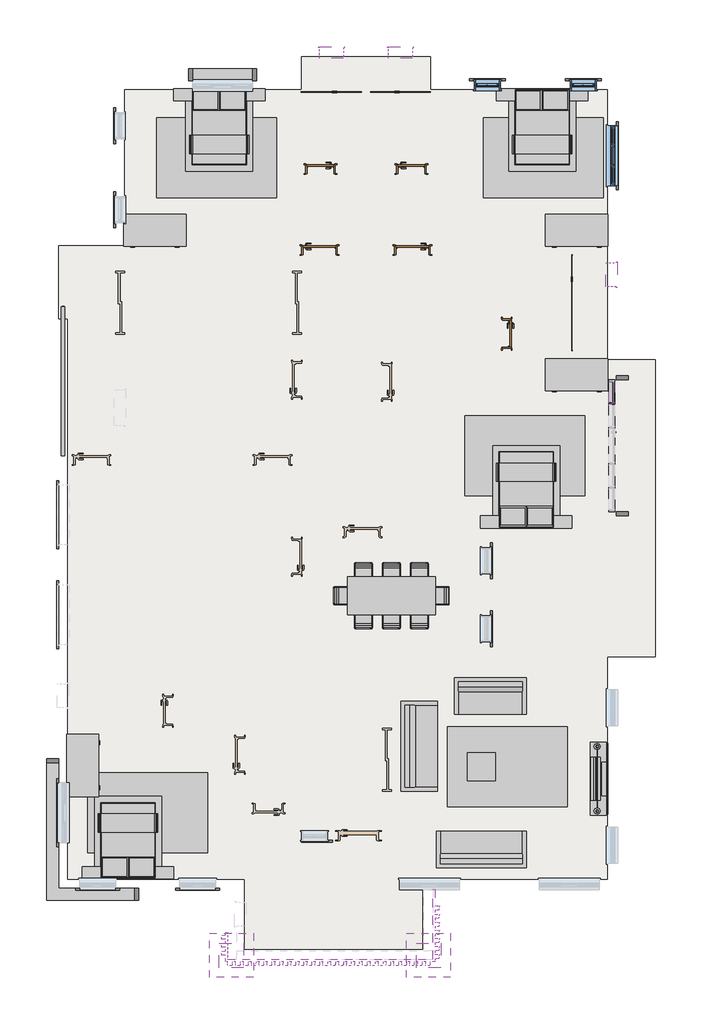
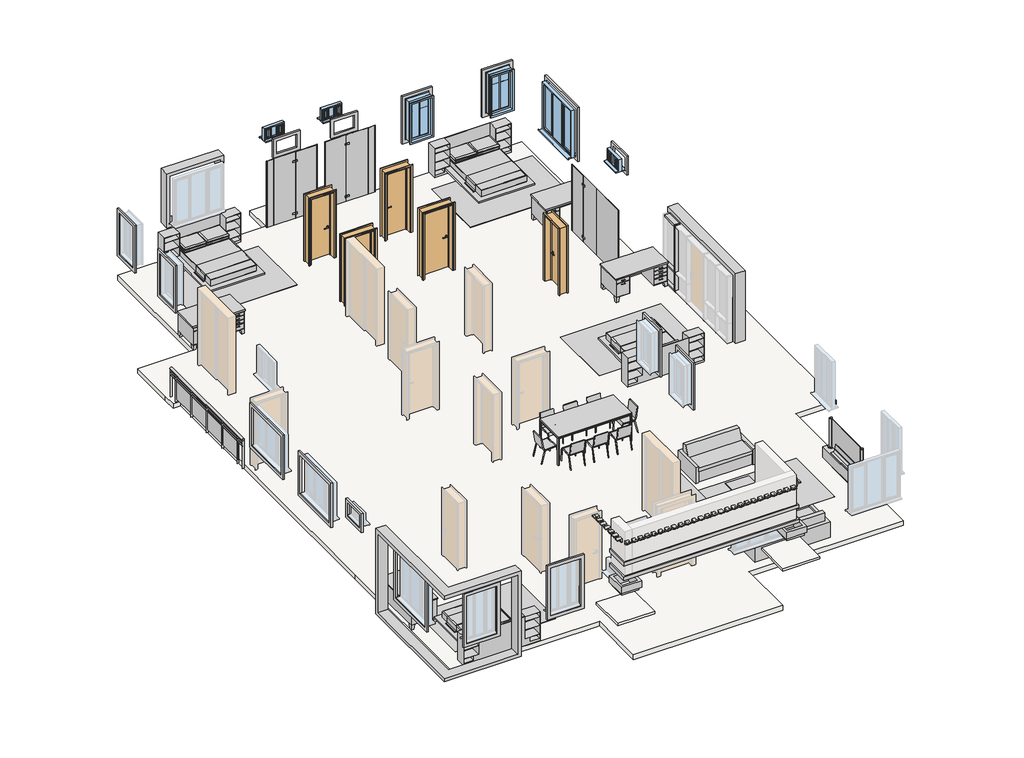
# One storey, part 2 of 2: 20 furniture elements, 6 members, 6 windows, 5 doors, 4 proxies, 3 flow terminals, 3 slabs, 1 railing.
"""IFC4 building model written with IfcOpenShell, lengths in millimetres."""

from ifc_helpers import new_model, si_unit, point, frame, origin, place, context, project, spatial, polyline, ellipse_curve, trimmed, outline, extrude, transform, mapped, element, save
from ifc_brep_helpers import plane_surface, extruded_surface, advanced_brep
from components import bed_6467_bed_6467_bd858abb, doors_intsgl_927b0b89, doors_intsgl_1caea894, doors_intsgl_900mm_doors_1c9cf9a6, doors_intsgl_900mm_doors_d21b38ee, hpl_shower_screen_rad_shower_screen_cut_corner_864de885, hpl_shower_screen_rad_shower_screen_cut_corner_ba801a97, hpl_shower_screen_rad_shower_screen_cut_corner_606f97bc, furniture_061ed33e, furniture_47c73875, furniture_703849cf, furniture_c31c7c6f, furniture_b53a9923, furniture_b3e58817, furniture_1e63cb50, casework_1_casework_1_62078cb6, casework_10_casework_10_bcdbd455, casework_3_casework_1_4875a9a3, casework_7_casework_7_7bbf8f76, casework_9_casework_9_0ee90f3f, entertainment_center_1_entertainment_center_18172_277d4ec1, m_desk_1525_x_762mm_student_8f660baf, rug1_rug_774cf3d5, rectangular_mullion_50_x_150mm_5b5377e9, rectangular_mullion_50_x_150mm_de2b7ee4, rectangular_mullion_50_x_150mm_8a69f4a4, rectangular_mullion_50_x_150mm_63369cdd, rectangular_mullion_50_x_150mm_c6835c94, tpl_plain_1500mm_wind_d4a9cd4c, tpl_plain_600mm_window_e9a44080, yu_window_casement_600x1200_84df8a12

model = new_model("IFC4")

# Units and contexts
model_context = context("Model", 3, world=origin())
ifc_project = project(units=[si_unit("LENGTHUNIT", "METRE", prefix="MILLI")], contexts=[model_context])

# Site, building, storey
site = spatial("IfcSite", under=ifc_project)
building = spatial("IfcBuilding", under=site)
storey = spatial("IfcBuildingStorey", under=building, Elevation=450.0)

# Proxies
placement = place(None, origin())
bed_6467_bed_6467_shape = bed_6467_bed_6467_bd858abb(model_context)
element("IfcBuildingElementProxy", 1, Name="BED_6467 : BED_6467", ObjectType="BED_6467 : BED_6467", at=placement, inside=storey, context=model_context, shape_type="MappedRepresentation", body=[
    mapped(bed_6467_bed_6467_shape, transform((-2061.7953966, 8065.8070837, 450.0), x_axis=(1.0, 0.0, 0.0), y_axis=(0.0, 1.0, 0.0), z_axis=(0.0, 0.0, 1.0))),
])
element("IfcBuildingElementProxy", 2, Name="BED_6467 : BED_6467", ObjectType="BED_6467 : BED_6467", at=placement, inside=storey, context=model_context, shape_type="MappedRepresentation", body=[
    mapped(bed_6467_bed_6467_shape, transform((6013.2046034, 8065.8070837, 450.0), x_axis=(1.0, 0.0, 0.0), y_axis=(0.0, 1.0, 0.0), z_axis=(0.0, 0.0, 1.0))),
])
element("IfcBuildingElementProxy", 3, Name="BED_6467 : BED_6467", ObjectType="BED_6467 : BED_6467", at=placement, inside=storey, context=model_context, shape_type="MappedRepresentation", body=[
    mapped(bed_6467_bed_6467_shape, transform((-4401.7953966, -10035.969736, 450.0), x_axis=(-1.0, 0.0, 0.0), y_axis=(0.0, -1.0, 0.0), z_axis=(0.0, 0.0, 1.0))),
])
element("IfcBuildingElementProxy", 4, Name="BED_6467 : BED_6467", ObjectType="BED_6467 : BED_6467", at=placement, inside=storey, context=model_context, shape_type="MappedRepresentation", body=[
    mapped(bed_6467_bed_6467_shape, transform((5556.3452648, -1269.6196108, 450.0), x_axis=(-1.0, 0.0, 0.0), y_axis=(0.0, -1.0, 0.0), z_axis=(0.0, 0.0, 1.0))),
])

# Doors
doors_intsgl_shape = doors_intsgl_927b0b89(model_context)
element("IfcDoor", 5, ObjectType="Doors_IntSgl", at=placement, inside=storey, context=model_context, shape_type="MappedRepresentation", body=[
    mapped(doors_intsgl_shape, transform((438.2046034, 6878.3070837, 450.0), x_axis=(-1.0, 0.0, 0.0), y_axis=(0.0, -1.0, 0.0), z_axis=(0.0, 0.0, 1.0))),
])
doors_intsgl_2_shape = doors_intsgl_1caea894(model_context)
element("IfcDoor", 6, ObjectType="Doors_IntSgl", at=placement, inside=storey, context=model_context, shape_type="MappedRepresentation", body=[
    mapped(doors_intsgl_2_shape, transform((2713.2046034, 6878.3070837, 450.0), x_axis=(1.0, 0.0, 0.0), y_axis=(0.0, 1.0, 0.0), z_axis=(0.0, 0.0, 1.0))),
])
element("IfcDoor", 7, ObjectType="Doors_IntSgl", at=placement, inside=storey, context=model_context, shape_type="MappedRepresentation", body=[
    mapped(doors_intsgl_2_shape, transform((5100.7046034, 2765.8070837, 450.0), x_axis=(0.0, -1.0, 0.0), y_axis=(1.0, 0.0, 0.0), z_axis=(0.0, 0.0, 1.0))),
])
doors_intsgl_900mm_doors_shape = doors_intsgl_900mm_doors_1c9cf9a6(model_context)
element("IfcDoor", 8, ObjectType="Doors_IntSgl : 900mm DOORS", at=placement, inside=storey, context=model_context, shape_type="MappedRepresentation", body=[
    mapped(doors_intsgl_900mm_doors_shape, transform((413.2046034, 4853.3070837, 450.0), x_axis=(1.0, 0.0, 0.0), y_axis=(0.0, 1.0, 0.0), z_axis=(0.0, 0.0, 1.0))),
])
doors_intsgl_900mm_doors_2_shape = doors_intsgl_900mm_doors_d21b38ee(model_context)
element("IfcDoor", 9, ObjectType="Doors_IntSgl : 900mm DOORS", at=placement, inside=storey, context=model_context, shape_type="MappedRepresentation", body=[
    mapped(doors_intsgl_900mm_doors_2_shape, transform((2738.2046034, 4853.3070837, 450.0), x_axis=(-1.0, 0.0, 0.0), y_axis=(0.0, -1.0, 0.0), z_axis=(0.0, 0.0, 1.0))),
])

# Flow terminals
hpl_shower_screen_rad_shower_screen_cut_corner_shape = hpl_shower_screen_rad_shower_screen_cut_corner_864de885(model_context)
element("IfcFlowTerminal", 10, ObjectType="HPL Shower Screen : RAD Shower Screen - cut corner", at=placement, inside=storey, context=model_context, shape_type="MappedRepresentation", body=[
    mapped(hpl_shower_screen_rad_shower_screen_cut_corner_shape, transform((2329.87127, 8790.8070837, 450.0), x_axis=(0.0, 1.0, 0.0), y_axis=(-1.0, 0.0, 0.0), z_axis=(0.0, 0.0, 1.0))),
])
hpl_shower_screen_rad_shower_screen_cut_corner_2_shape = hpl_shower_screen_rad_shower_screen_cut_corner_ba801a97(model_context)
element("IfcFlowTerminal", 11, ObjectType="HPL Shower Screen : RAD Shower Screen - cut corner", at=placement, inside=storey, context=model_context, shape_type="MappedRepresentation", body=[
    mapped(hpl_shower_screen_rad_shower_screen_cut_corner_2_shape, transform((6713.2046034, 4140.8070837, 450.0), x_axis=(1.0, 0.0, 0.0), y_axis=(0.0, 1.0, 0.0), z_axis=(0.0, 0.0, 1.0))),
])
hpl_shower_screen_rad_shower_screen_cut_corner_3_shape = hpl_shower_screen_rad_shower_screen_cut_corner_606f97bc(model_context)
element("IfcFlowTerminal", 12, ObjectType="HPL Shower Screen : RAD Shower Screen - cut corner", at=placement, inside=storey, context=model_context, shape_type="MappedRepresentation", body=[
    mapped(hpl_shower_screen_rad_shower_screen_cut_corner_3_shape, transform((808.5072032, 8790.8070837, 450.0), x_axis=(0.0, 1.0, 0.0), y_axis=(-1.0, 0.0, 0.0), z_axis=(0.0, 0.0, 1.0))),
])

# Furniture
furniture_shape = furniture_061ed33e(model_context)
element("IfcFurniture", 13, at=placement, inside=storey, context=model_context, shape_type="MappedRepresentation", body=[
    mapped(furniture_shape, transform((4463.2046034, -8059.1929163, 450.0), x_axis=(1.0, 0.0, 0.0), y_axis=(0.0, 1.0, 0.0), z_axis=(0.0, 0.0, 1.0))),
])
furniture_2_shape = furniture_47c73875(model_context)
element("IfcFurniture", 14, at=placement, inside=storey, context=model_context, shape_type="MappedRepresentation", body=[
    mapped(furniture_2_shape, transform((2458.2046034, -7622.8929163, 450.0), x_axis=(0.0, 1.0, 0.0), y_axis=(-1.0, 0.0, 0.0), z_axis=(0.0, 0.0, 1.0))),
])
element("IfcFurniture", 15, at=placement, inside=storey, context=model_context, shape_type="MappedRepresentation", body=[
    mapped(furniture_2_shape, transform((4539.4046034, -10581.6929163, 450.0), x_axis=(-1.0, 0.0, 0.0), y_axis=(0.0, -1.0, 0.0), z_axis=(0.0, 0.0, 1.0))),
])
furniture_3_shape = furniture_703849cf(model_context)
element("IfcFurniture", 16, at=placement, inside=storey, context=model_context, shape_type="MappedRepresentation", body=[
    mapped(furniture_3_shape, transform((4612.0046034, -5834.1929163, 450.0), x_axis=(1.0, 0.0, 0.0), y_axis=(0.0, 1.0, 0.0), z_axis=(0.0, 0.0, 1.0))),
])
furniture_4_shape = furniture_c31c7c6f(model_context)
furniture_5_shape = furniture_b53a9923(model_context)
furniture_6_shape = furniture_b3e58817(model_context)
furniture_7_shape = furniture_1e63cb50(model_context)
element("IfcFurniture", 17, at=placement, inside=storey, context=model_context, shape_type="MappedRepresentation", body=[
    mapped(furniture_4_shape, transform((2699.7692743, -3784.1929163, 450.0), x_axis=(1.0, 0.0, 0.0), y_axis=(0.0, 1.0, 0.0), z_axis=(0.0, 0.0, 1.0))),
    mapped(furniture_5_shape, transform((2699.7692743, -3784.1929163, 450.0), x_axis=(1.0, 0.0, 0.0), y_axis=(0.0, 1.0, 0.0), z_axis=(0.0, 0.0, 1.0))),
    mapped(furniture_6_shape, transform((2699.7692743, -3784.1929163, 450.0), x_axis=(1.0, 0.0, 0.0), y_axis=(0.0, 1.0, 0.0), z_axis=(0.0, 0.0, 1.0))),
    mapped(furniture_7_shape, transform((2699.7692743, -3784.1929163, 450.0), x_axis=(1.0, 0.0, 0.0), y_axis=(0.0, 1.0, 0.0), z_axis=(0.0, 0.0, 1.0))),
])
casework_1_casework_1_shape = casework_1_casework_1_62078cb6(model_context)
element("IfcFurniture", 18, ObjectType="Casework 1 : Casework 1", at=placement, inside=storey, context=model_context, shape_type="MappedRepresentation", body=[
    mapped(casework_1_casework_1_shape, transform((-29.8857753, 1024.70238, -675.0), x_axis=(1.0, 0.0, 0.0), y_axis=(0.0, 1.0, 0.0), z_axis=(0.0, 0.0, 1.0))),
])
casework_10_casework_10_shape = casework_10_casework_10_bcdbd455(model_context)
element("IfcFurniture", 19, ObjectType="Casework 10 : Casework 10", at=placement, inside=storey, context=model_context, shape_type="MappedRepresentation", body=[
    mapped(casework_10_casework_10_shape, transform((0.0, 0.0, 0.0), x_axis=(1.0, 0.0, 0.0), y_axis=(0.0, 1.0, 0.0), z_axis=(0.0, 0.0, 1.0))),
])
casework_3_casework_1_shape = casework_3_casework_1_4875a9a3(model_context)
element("IfcFurniture", 20, ObjectType="Casework 3 : Casework 1", at=placement, inside=storey, context=model_context, shape_type="MappedRepresentation", body=[
    mapped(casework_3_casework_1_shape, transform((-29.8857753, 1024.70238, -675.0), x_axis=(1.0, 0.0, 0.0), y_axis=(0.0, 1.0, 0.0), z_axis=(0.0, 0.0, 1.0))),
])
casework_7_casework_7_shape = casework_7_casework_7_7bbf8f76(model_context)
element("IfcFurniture", 21, ObjectType="Casework 7 : Casework 7", at=placement, inside=storey, context=model_context, shape_type="MappedRepresentation", body=[
    mapped(casework_7_casework_7_shape, transform((0.0, 0.0, 0.0), x_axis=(1.0, 0.0, 0.0), y_axis=(0.0, 1.0, 0.0), z_axis=(0.0, 0.0, 1.0))),
])
casework_9_casework_9_shape = casework_9_casework_9_0ee90f3f(model_context)
element("IfcFurniture", 22, ObjectType="Casework 9 : Casework 9", at=placement, inside=storey, context=model_context, shape_type="MappedRepresentation", body=[
    mapped(casework_9_casework_9_shape, transform((0.0, 0.0, 0.0), x_axis=(1.0, 0.0, 0.0), y_axis=(0.0, 1.0, 0.0), z_axis=(0.0, 0.0, 1.0))),
])
entertainment_center_1_entertainment_center_18172_shape = entertainment_center_1_entertainment_center_18172_277d4ec1(model_context)
element("IfcFurniture", 23, ObjectType="Entertainment_Center_1 : Entertainment_Center_18172", at=placement, inside=storey, context=model_context, shape_type="MappedRepresentation", body=[
    mapped(entertainment_center_1_entertainment_center_18172_shape, transform((7188.2046034, -8359.1929163, 450.0), x_axis=(0.0, 1.0, 0.0), y_axis=(-1.0, 0.0, 0.0), z_axis=(0.0, 0.0, 1.0))),
])
m_desk_1525_x_762mm_student_shape = m_desk_1525_x_762mm_student_8f660baf(model_context)
element("IfcFurniture", 24, ObjectType="M_Desk : 1525 x 762mm Student", at=placement, inside=storey, context=model_context, shape_type="MappedRepresentation", body=[
    mapped(m_desk_1525_x_762mm_student_shape, transform((-4461.2953966, 4965.8070837, 450.0), x_axis=(1.0, 0.0, 0.0), y_axis=(0.0, 1.0, 0.0), z_axis=(0.0, 0.0, 1.0))),
])
element("IfcFurniture", 25, ObjectType="M_Desk : 1525 x 762mm Student", at=placement, inside=storey, context=model_context, shape_type="MappedRepresentation", body=[
    mapped(m_desk_1525_x_762mm_student_shape, transform((6088.7046034, 4965.8070837, 450.0), x_axis=(1.0, 0.0, 0.0), y_axis=(0.0, 1.0, 0.0), z_axis=(0.0, 0.0, 1.0))),
])
element("IfcFurniture", 26, ObjectType="M_Desk : 1525 x 762mm Student", at=placement, inside=storey, context=model_context, shape_type="MappedRepresentation", body=[
    mapped(m_desk_1525_x_762mm_student_shape, transform((6088.7046034, 1353.8070837, 450.0), x_axis=(1.0, 0.0, 0.0), y_axis=(0.0, 1.0, 0.0), z_axis=(0.0, 0.0, 1.0))),
])
element("IfcFurniture", 27, ObjectType="M_Desk : 1525 x 762mm Student", at=placement, inside=storey, context=model_context, shape_type="MappedRepresentation", body=[
    mapped(m_desk_1525_x_762mm_student_shape, transform((-5124.7953966, -8783.6929163, 450.0), x_axis=(0.0, 1.0, 0.0), y_axis=(-1.0, 0.0, 0.0), z_axis=(0.0, 0.0, 1.0))),
])
rug1_rug_shape = rug1_rug_774cf3d5(model_context)
element("IfcFurniture", 28, ObjectType="Rug1 : Rug", at=placement, inside=storey, context=model_context, shape_type="MappedRepresentation", body=[
    mapped(rug1_rug_shape, transform((-2161.7953966, 7165.8070837, 450.0), x_axis=(1.0, 0.0, 0.0), y_axis=(0.0, 1.0, 0.0), z_axis=(0.0, 0.0, 1.0))),
])
element("IfcFurniture", 29, ObjectType="Rug1 : Rug", at=placement, inside=storey, context=model_context, shape_type="MappedRepresentation", body=[
    mapped(rug1_rug_shape, transform((6013.2046034, 7165.8070837, 450.0), x_axis=(1.0, 0.0, 0.0), y_axis=(0.0, 1.0, 0.0), z_axis=(0.0, 0.0, 1.0))),
])
element("IfcFurniture", 30, ObjectType="Rug1 : Rug", at=placement, inside=storey, context=model_context, shape_type="MappedRepresentation", body=[
    mapped(rug1_rug_shape, transform((-3886.7953966, -9209.1929163, 450.0), x_axis=(1.0, 0.0, 0.0), y_axis=(0.0, 1.0, 0.0), z_axis=(0.0, 0.0, 1.0))),
])
element("IfcFurniture", 31, ObjectType="Rug1 : Rug", at=placement, inside=storey, context=model_context, shape_type="MappedRepresentation", body=[
    mapped(rug1_rug_shape, transform((5556.3452648, -284.1929163, 450.0), x_axis=(1.0, 0.0, 0.0), y_axis=(0.0, 1.0, 0.0), z_axis=(0.0, 0.0, 1.0))),
])
element("IfcFurniture", 32, ObjectType="Rug1 : Rug", at=placement, inside=storey, context=model_context, shape_type="MappedRepresentation", body=[
    mapped(rug1_rug_shape, transform((5113.2046034, -8059.1929163, 450.0), x_axis=(1.0, 0.0, 0.0), y_axis=(0.0, 1.0, 0.0), z_axis=(0.0, 0.0, 1.0))),
])

# Members
rectangular_mullion_50_x_150mm_shape = rectangular_mullion_50_x_150mm_5b5377e9(model_context)
element("IfcMember", 33, ObjectType="Rectangular Mullion : 50 x 150mm", at=placement, inside=storey, context=model_context, shape_type="MappedRepresentation", body=[
    mapped(rectangular_mullion_50_x_150mm_shape, transform((7725.7046034, 1040.8070837, 2550.0), x_axis=(0.0, 0.0, 1.0), y_axis=(-1.0, 0.0, 0.0), z_axis=(0.0, -1.0, 0.0))),
])
element("IfcMember", 34, ObjectType="Rectangular Mullion : 50 x 150mm", at=placement, inside=storey, context=model_context, shape_type="MappedRepresentation", body=[
    mapped(rectangular_mullion_50_x_150mm_shape, transform((7725.7046034, 1565.8070837, 450.0), x_axis=(0.0, 0.0, -1.0), y_axis=(-1.0, 0.0, 0.0), z_axis=(0.0, 1.0, 0.0))),
])
rectangular_mullion_50_x_150mm_2_shape = rectangular_mullion_50_x_150mm_de2b7ee4(model_context)
element("IfcMember", 35, ObjectType="Rectangular Mullion : 50 x 150mm", at=placement, inside=storey, context=model_context, shape_type="MappedRepresentation", body=[
    mapped(rectangular_mullion_50_x_150mm_2_shape, transform((7725.7046034, 1015.8070837, 450.0), x_axis=(0.0, -1.0, 0.0), y_axis=(-1.0, 0.0, 0.0), z_axis=(0.0, 0.0, -1.0))),
])
rectangular_mullion_50_x_150mm_3_shape = rectangular_mullion_50_x_150mm_8a69f4a4(model_context)
element("IfcMember", 36, ObjectType="Rectangular Mullion : 50 x 150mm", at=placement, inside=storey, context=model_context, shape_type="MappedRepresentation", body=[
    mapped(rectangular_mullion_50_x_150mm_3_shape, transform((7725.7046034, 1040.8070837, 1060.0), x_axis=(0.0, 0.0, 1.0), y_axis=(-1.0, 0.0, 0.0), z_axis=(0.0, -1.0, 0.0))),
])
rectangular_mullion_50_x_150mm_4_shape = rectangular_mullion_50_x_150mm_63369cdd(model_context)
element("IfcMember", 37, ObjectType="Rectangular Mullion : 50 x 150mm", at=placement, inside=storey, context=model_context, shape_type="MappedRepresentation", body=[
    mapped(rectangular_mullion_50_x_150mm_4_shape, transform((7725.7046034, 1015.8070837, 1060.0), x_axis=(0.0, -1.0, 0.0), y_axis=(-1.0, 0.0, 0.0), z_axis=(0.0, 0.0, -1.0))),
])
rectangular_mullion_50_x_150mm_5_shape = rectangular_mullion_50_x_150mm_c6835c94(model_context)
element("IfcMember", 38, ObjectType="Rectangular Mullion : 50 x 150mm", at=placement, inside=storey, context=model_context, shape_type="MappedRepresentation", body=[
    mapped(rectangular_mullion_50_x_150mm_5_shape, transform((7725.7046034, 1615.8070837, 1060.0), x_axis=(0.0, 1.0, 0.0), y_axis=(-1.0, 0.0, 0.0), z_axis=(0.0, 0.0, 1.0))),
])

# Railing
element("IfcRailing", 39, ObjectType="Glass Panel - Bottom Fill", at=placement, inside=storey, context=model_context, shape_type="SolidModel", body=[
    advanced_brep(
    [(-6038.6861618, -284.1929163, 1350.0), (-5958.6861618, -284.1929163, 1350.0), (-6038.6861618, 3440.8070837, 1350.0), (-5958.6861618, 3440.8070837, 1350.0)],
    [
        (0, 1, ellipse_curve(frame((-5998.6861618, -284.1929163, 1350.0), z_axis=(0.0, -1.0, 0.0), x_axis=(1.0, 0.0, 0.0)), 40.0, 30.0)),
        (1, 0, ellipse_curve(frame((-5998.6861618, -284.1929163, 1350.0), z_axis=(0.0, -1.0, 0.0), x_axis=(1.0, 0.0, 0.0)), 40.0, 30.0)),
        (2, 3, ellipse_curve(frame((-5998.6861618, 3440.8070837, 1350.0), z_axis=(0.0, 1.0, 0.0), x_axis=(1.0, 0.0, 0.0)), 40.0, 30.0)),
        (3, 2, ellipse_curve(frame((-5998.6861618, 3440.8070837, 1350.0), z_axis=(0.0, 1.0, 0.0), x_axis=(1.0, 0.0, 0.0)), 40.0, 30.0)),
        (0, 2),
        (3, 1),
    ],
    [
        plane_surface(frame((-5998.6861618, -284.1929163, 1350.0), z_axis=(0.0, -1.0, 0.0), x_axis=(0.0, 0.0, 1.0))),
        plane_surface(frame((-5998.6861618, 3440.8070837, 1350.0), z_axis=(0.0, 1.0, 0.0), x_axis=(0.0, 0.0, 1.0))),
        extruded_surface(trimmed(ellipse_curve(frame((-5998.6861618, 3440.8070837, 1350.0), z_axis=(0.0, -1.0, 0.0), x_axis=(1.0, 0.0, 0.0)), 40.0, 30.0), [point((-6038.6861618, 3440.8070837, 1350.0))], [point((-5958.6861618, 3440.8070837, 1350.0))], True, "CARTESIAN"), (0.0, -3725.0, 0.0), 3725.0),
        extruded_surface(trimmed(ellipse_curve(frame((-5998.6861618, 3440.8070837, 1350.0), z_axis=(0.0, -1.0, 0.0), x_axis=(1.0, 0.0, 0.0)), 40.0, 30.0), [point((-5958.6861618, 3440.8070837, 1350.0))], [point((-6038.6861618, 3440.8070837, 1350.0))], True, "CARTESIAN"), (0.0, -3725.0, 0.0), 3725.0),
    ],
    [
        (0, [[1, 2]]),
        (1, [[3, 4]]),
        (2, [[-1, 5, -4, 6]]),
        (3, [[-2, -6, -3, -5]]),
    ],
),
    extrude(outline(polyline([(-5989.2953966, -284.1929163), (-6009.2953966, -284.1929163), (-6009.2953966, 3440.8070837), (-5989.2953966, 3440.8070837), (-5989.2953966, -284.1929163)])), frame((0.0, 0.0, 1230.0), z_axis=(0.0, 0.0, 1.0), x_axis=(1.0, 0.0, 0.0)), (0.0, 0.0, 1.0), 20.0),
    extrude(outline(polyline([(-5989.2953966, -284.1929163), (-6009.2953966, -284.1929163), (-6009.2953966, 3440.8070837), (-5989.2953966, 3440.8070837), (-5989.2953966, -284.1929163)])), frame((0.0, 0.0, 1130.0), z_axis=(0.0, 0.0, 1.0), x_axis=(1.0, 0.0, 0.0)), (0.0, 0.0, 1.0), 20.0),
    extrude(outline(polyline([(-6024.2953966, 3172.3070837), (-6024.2953966, 3184.3070837), (-5974.2953966, 3184.3070837), (-5974.2953966, 3172.3070837), (-6024.2953966, 3172.3070837)])), frame((0.0, 0.0, 450.0), z_axis=(0.0, 0.0, 1.0), x_axis=(1.0, 0.0, 0.0)), (0.0, 0.0, 1.0), 870.0),
    extrude(outline(polyline([(-5997.5705865, 2378.3070837), (-5997.5705865, 3178.3070837), (-5992.5705865, 3178.3070837), (-5992.5705865, 2378.3070837), (-5997.5705865, 2378.3070837)])), frame((0.0, 0.0, 550.0), z_axis=(0.0, 0.0, 1.0), x_axis=(1.0, 0.0, 0.0)), (0.0, 0.0, 1.0), 580.0),
    extrude(outline(polyline([(-6024.2953966, 2372.3070837), (-6024.2953966, 2384.3070837), (-5974.2953966, 2384.3070837), (-5974.2953966, 2372.3070837), (-6024.2953966, 2372.3070837)])), frame((0.0, 0.0, 450.0), z_axis=(0.0, 0.0, 1.0), x_axis=(1.0, 0.0, 0.0)), (0.0, 0.0, 1.0), 870.0),
    extrude(outline(polyline([(-5997.5705865, 1578.3070837), (-5997.5705865, 2378.3070837), (-5992.5705865, 2378.3070837), (-5992.5705865, 1578.3070837), (-5997.5705865, 1578.3070837)])), frame((0.0, 0.0, 550.0), z_axis=(0.0, 0.0, 1.0), x_axis=(1.0, 0.0, 0.0)), (0.0, 0.0, 1.0), 580.0),
    extrude(outline(polyline([(-6024.2953966, 1572.3070837), (-6024.2953966, 1584.3070837), (-5974.2953966, 1584.3070837), (-5974.2953966, 1572.3070837), (-6024.2953966, 1572.3070837)])), frame((0.0, 0.0, 450.0), z_axis=(0.0, 0.0, 1.0), x_axis=(1.0, 0.0, 0.0)), (0.0, 0.0, 1.0), 870.0),
    extrude(outline(polyline([(-5997.5705865, 778.3070837), (-5997.5705865, 1578.3070837), (-5992.5705865, 1578.3070837), (-5992.5705865, 778.3070837), (-5997.5705865, 778.3070837)])), frame((0.0, 0.0, 550.0), z_axis=(0.0, 0.0, 1.0), x_axis=(1.0, 0.0, 0.0)), (0.0, 0.0, 1.0), 580.0),
    extrude(outline(polyline([(-6024.2953966, 772.3070837), (-6024.2953966, 784.3070837), (-5974.2953966, 784.3070837), (-5974.2953966, 772.3070837), (-6024.2953966, 772.3070837)])), frame((0.0, 0.0, 450.0), z_axis=(0.0, 0.0, 1.0), x_axis=(1.0, 0.0, 0.0)), (0.0, 0.0, 1.0), 870.0),
    extrude(outline(polyline([(-5997.5705865, -21.6929163), (-5997.5705865, 778.3070837), (-5992.5705865, 778.3070837), (-5992.5705865, -21.6929163), (-5997.5705865, -21.6929163)])), frame((0.0, 0.0, 550.0), z_axis=(0.0, 0.0, 1.0), x_axis=(1.0, 0.0, 0.0)), (0.0, 0.0, 1.0), 580.0),
    extrude(outline(polyline([(-6024.2953966, -27.6929163), (-6024.2953966, -15.6929163), (-5974.2953966, -15.6929163), (-5974.2953966, -27.6929163), (-6024.2953966, -27.6929163)])), frame((0.0, 0.0, 450.0), z_axis=(0.0, 0.0, 1.0), x_axis=(1.0, 0.0, 0.0)), (0.0, 0.0, 1.0), 870.0),
    extrude(outline(polyline([(-6024.2953966, 3432.8070837), (-6024.2953966, 3444.8070837), (-5974.2953966, 3444.8070837), (-5974.2953966, 3432.8070837), (-6024.2953966, 3432.8070837)])), frame((0.0, 0.0, 450.0), z_axis=(0.0, 0.0, 1.0), x_axis=(1.0, 0.0, 0.0)), (0.0, 0.0, 1.0), 870.0),
    extrude(outline(polyline([(-6024.2953966, -288.1929163), (-6024.2953966, -276.1929163), (-5974.2953966, -276.1929163), (-5974.2953966, -288.1929163), (-6024.2953966, -288.1929163)])), frame((0.0, 0.0, 450.0), z_axis=(0.0, 0.0, 1.0), x_axis=(1.0, 0.0, 0.0)), (0.0, 0.0, 1.0), 870.0),
])

# Slabs
element("IfcSlab", 40, ObjectType="6\" floor", at=placement, inside=storey, context=model_context, shape_type="SweptSolid", body=[
    extrude(outline(polyline([(-36.7953966, 8865.8070837), (-36.7953966, 9690.8070837), (3188.2046034, 9690.8070837), (3188.2046034, 8865.8070837), (7613.2046034, 8865.8070837), (7613.2046034, 2115.8070837), (8813.2046034, 2115.8070837), (8813.2046034, -5309.1929163), (7613.2046034, -5309.1929163), (7613.2046034, -10871.6929163), (2993.2046034, -10871.6929163), (2993.2046034, -12624.1929163), (-1461.7953966, -12624.1929163), (-1461.7953966, -10871.6929163), (-5886.7953966, -10871.6929163), (-5886.7953966, -5894.7974899), (-5886.7953966, 3140.8070837), (-6111.7953966, 3140.8070837), (-6111.7953966, 3537.9094476), (-6111.7953966, 4965.8070837), (-4461.7953966, 4965.8070837), (-4461.7953966, 8865.8070837), (-36.7953966, 8865.8070837)])), frame((0.0, 0.0, 300.0), z_axis=(0.0, 0.0, 1.0), x_axis=(1.0, 0.0, 0.0)), (0.0, 0.0, 1.0), 150.0),
])
element("IfcSlab", 41, ObjectType="75mm", at=placement, inside=storey, context=model_context, shape_type="SweptSolid", body=[
    extrude(outline(polyline([(-1236.7953966, -12224.1929163), (-1236.7953966, -13324.1929163), (-2336.7953966, -13324.1929163), (-2336.7953966, -12224.1929163), (-1236.7953966, -12224.1929163)])), frame((0.0, 0.0, 2100.0), z_axis=(0.0, 0.0, 1.0), x_axis=(1.0, 0.0, 0.0)), (0.0, 0.0, 1.0), 75.0),
])
element("IfcSlab", 42, ObjectType="75mm", at=placement, inside=storey, context=model_context, shape_type="SweptSolid", body=[
    extrude(outline(polyline([(3693.2046034, -12224.1929163), (3693.2046034, -13324.1929163), (2593.2046034, -13324.1929163), (2593.2046034, -12224.1929163), (3693.2046034, -12224.1929163)])), frame((0.0, 0.0, 2100.0), z_axis=(0.0, 0.0, 1.0), x_axis=(1.0, 0.0, 0.0)), (0.0, 0.0, 1.0), 75.0),
])

# Windows
tpl_plain_1500mm_wind_shape = tpl_plain_1500mm_wind_d4a9cd4c(model_context)
element("IfcWindow", 43, ObjectType="Tpl Plain : 1500mm wind", at=placement, inside=storey, context=model_context, shape_type="MappedRepresentation", body=[
    mapped(tpl_plain_1500mm_wind_shape, transform((7717.2480355, 6690.8070837, 450.0), x_axis=(0.0, -1.0, 0.0), y_axis=(1.0, 0.0, 0.0), z_axis=(0.0, 0.0, 1.0))),
])
tpl_plain_600mm_window_shape = tpl_plain_600mm_window_e9a44080(model_context)
element("IfcWindow", 44, ObjectType="Tpl Plain : 600mm window", at=placement, inside=storey, context=model_context, shape_type="MappedRepresentation", body=[
    mapped(tpl_plain_600mm_window_shape, transform((2063.2046034, 9811.7636515, 450.0), x_axis=(-1.0, 0.0, 0.0), y_axis=(0.0, -1.0, 0.0), z_axis=(0.0, 0.0, 1.0))),
])
element("IfcWindow", 45, ObjectType="Tpl Plain : 600mm window", at=placement, inside=storey, context=model_context, shape_type="MappedRepresentation", body=[
    mapped(tpl_plain_600mm_window_shape, transform((7734.1611712, 4615.8070837, 450.0), x_axis=(0.0, 1.0, 0.0), y_axis=(-1.0, 0.0, 0.0), z_axis=(0.0, 0.0, 1.0))),
])
element("IfcWindow", 46, ObjectType="Tpl Plain : 600mm window", at=placement, inside=storey, context=model_context, shape_type="MappedRepresentation", body=[
    mapped(tpl_plain_600mm_window_shape, transform((338.2046034, 9811.7636515, 450.0), x_axis=(-1.0, 0.0, 0.0), y_axis=(0.0, -1.0, 0.0), z_axis=(0.0, 0.0, 1.0))),
])
yu_window_casement_600x1200_shape = yu_window_casement_600x1200_84df8a12(model_context)
element("IfcWindow", 47, ObjectType="Yu_Window : Casement 600x1200", at=placement, inside=storey, context=model_context, shape_type="MappedRepresentation", body=[
    mapped(yu_window_casement_600x1200_shape, transform((4613.2046034, 8978.3070837, 990.0), x_axis=(-1.0, 0.0, 0.0), y_axis=(0.0, -1.0, 0.0), z_axis=(0.0, 0.0, 1.0))),
])
element("IfcWindow", 48, ObjectType="Yu_Window : Casement 600x1200", at=placement, inside=storey, context=model_context, shape_type="MappedRepresentation", body=[
    mapped(yu_window_casement_600x1200_shape, transform((7013.2046034, 8978.3070837, 990.0), x_axis=(-1.0, 0.0, 0.0), y_axis=(0.0, -1.0, 0.0), z_axis=(0.0, 0.0, 1.0))),
])

save(model, "model.ifc")

# Revit data of these elements
# Type "BED_6467 : BED_6467"
#   Sheets [instance default] = Sheets
#   Pillow Set 2 [instance default] = Pillow 2
#   Pillow Set 1 [instance default] = Pillow 1
#   FRAME [instance default] = frame
#   Default Elevation = 0
# Type "Doors_IntSgl"
#   Type Mark = "45"
#   Type Comments = "Internal Single"
#   Operation = "SingleSwingRight"
#   Manufacturer = "Revit"
#   Keynote = "L20"
#   Description = "Internal Single Door"
#   Analytic Construction = "Metal"
#   UnderCut = 8 mm
#   Tolerance = 2 mm
#   Thickness = 38 mm
#   Thermal Resistance (R) = 0.270117 (m²·K)/W
#   Structural Tolerance = 8 mm
#   StopDepth = 32 mm
#   Stop Thickness = 19 mm
#   Rough Width = 750 mm
#   Rough Height = 2100 mm
#   Height to Top Lock Rail = 1000 mm
#   Heat Transfer Coefficient (U) = 3.7021 W/(m²·K)
#   Handle Z Distance = 900 mm
#   Handle X Distance = 75 mm
#   Frame Thickness = 32 mm
#   Door Panel Width = 666 mm
#   Door Panel Thickness = 38 mm
#   Door Panel Offset = 0 mm
#   Height = 2100 mm
#   Width = 750 mm
#   Door Panel Height = 2050 mm
#   Architrave Setback = 5 mm
#   Vis - Ironmongery = yes
#   Define Thermal Properties by = 1
#   Material Ironmongery = Door - Handle
#   Material Frame = Door - Frame/Mullion (1)
#   Material Door = Door - Panel
#   Material Architrave = Door - Architrave
#   Visual Light Transmittance = 0
#   Solar Heat Gain Coefficient = 0
#   Function = (empty or 0)
#   Wall Closure = (empty or 0)
# Type "Doors_IntSgl : 900mm DOORS"
#   Type Mark = "46"
#   Type Comments = "Internal Single"
#   Operation = "SingleSwingRight"
#   Manufacturer = "Revit"
#   Keynote = "L20"
#   Description = "Internal Single Door"
#   Analytic Construction = "Metal"
#   UnderCut = 8 mm
#   Tolerance = 2 mm
#   Thickness = 38 mm
#   Thermal Resistance (R) = 0.270117 (m²·K)/W
#   Structural Tolerance = 8 mm
#   StopDepth = 32 mm
#   Stop Thickness = 19 mm
#   Rough Width = 900 mm
#   Rough Height = 2100 mm
#   Height to Top Lock Rail = 1000 mm
#   Heat Transfer Coefficient (U) = 3.7021 W/(m²·K)
#   Handle Z Distance = 1000 mm
#   Handle X Distance = 75 mm
#   Frame Thickness = 32 mm
#   Door Panel Width = 816 mm
#   Door Panel Thickness = 38 mm
#   Door Panel Offset = 0 mm
#   Height = 2100 mm
#   Width = 900 mm
#   Door Panel Height = 2050 mm
#   Architrave Setback = 5 mm
#   Vis - Ironmongery = yes
#   Define Thermal Properties by = 1
#   Material Ironmongery = Door - Handle
#   Material Frame = Door - Frame/Mullion (1)
#   Material Door = Door - Panel
#   Material Architrave = Door - Architrave
#   Visual Light Transmittance = 0
#   Solar Heat Gain Coefficient = 0
#   Function = (empty or 0)
#   Wall Closure = (empty or 0)
# Type "HPL Shower Screen : RAD Shower Screen - cut corner"
#   URL = "http://www.matki.co.uk/"
#   Model = "EPW1150 BESPOKE - 'Eauzone Plus' - left hand recess"
#   Manufacturer = "MATKI"
#   Description = "Shower screen - chamfered fixed panel"
#   Fixed panel width [instance default] = 296 mm
#   End Panel Width [instance default] = 100 mm
#   Door Width = 650 mm
#   Offset = 0 mm
#   Height = 2100 mm
#   Door [instance default] = yes
#   Default Elevation = 0
# Type
#   Default Elevation = 0
# Type
#   width = 2250 mm
#   seat height = 450 mm
#   height = 760 mm
#   depth = 910 mm
#   arm height = 500 mm
#   arm depth = 100 mm
#   Total Seat Room = 2050 mm
#   Seat Width = 683.333 mm
#   Seat Count = 3
#   Is Mark Visible = yes
#   seat material = Sofa seat
#   arm material = Sofa arm
#   Default Elevation = 0
#   Assembly Code = ""
# Type
#   width = 1800 mm
#   seat height = 450 mm
#   height = 760 mm
#   depth = 910 mm
#   arm height = 500 mm
#   arm depth = 100 mm
#   Total Seat Room = 1600 mm
#   Seat Width = 800 mm
#   Seat Count = 2
#   Is Mark Visible = yes
#   seat material = Sofa seat
#   arm material = Sofa arm
#   Default Elevation = 0
#   Assembly Code = ""
# Type
#   Stärke Tischplatte = 30 mm
#   Breite von Bein = 30 mm
#   Höhe = 900 mm
#   Länge = 2200 mm
#   Tiefe = 950 mm
#   Seitlicher Versatz Stuhlachse = 400 mm
#   Stühle vorn = yes
#   Stühle seitlich = yes
#   Im Vordergrund zeichnen [instance] = yes
#   Anzahl Stühle pro Seite = 3
#   2 Stühle zentriert = no
#   Tischgestell = none
#   Stuhlbeine = none
#   Default Elevation = 0
#   Assembly Code = ""
# Type "Entertainment_Center_1 : Entertainment_Center_18172"
#   TV Screen = tv screen
#   TV Material = Plastic, Opaque Black
#   Console Material = Plastic, Opaque White
#   Console Glass = Glass, Cast, Clear
#   Default Elevation = 0
# Type "M_Desk : 1525 x 762mm Student"
#   Depth = 762 mm
#   Height = 762 mm
#   Leg Height = 152 mm
#   Width = 1525 mm
#   Body Material = Laminate, Ivory, Matte
#   Handle/Leg Material = Steel, Chrome Plated
#   Top Material = Cherry
#   Default Elevation = 0
#   Assembly Code = ""
# Type "Rug1 : Rug"
#   boarder [instance default] = 100 mm
#   W [instance default] = 3000 mm
#   D [instance default] = 2000 mm
#   Boarder_2 [instance default] = no
#   main material [instance default] = Rug main
#   boarder material [instance default] = Rug Boarder
#   Default Elevation = 0
# Type "Rectangular Mullion : 50 x 150mm"
#   built-in parameter 1007304 = 0.492126 (stored number, unit not read)
#   built-in parameter 1007301 = 0.082021 (stored number, unit not read)
#   built-in parameter 1007300 = 0.082021 (stored number, unit not read)
# Type "Glass Panel - Bottom Fill"
#   built-in parameter 1008612 = 0.019685 (stored number, unit not read)
#   built-in parameter 1008611 = 0.019685 (stored number, unit not read)
#   built-in parameter 1008609 = 0.902231 (stored number, unit not read)
#   built-in parameter 1008604 = 0.19685 (stored number, unit not read)
#   built-in parameter 1008603 = 0.164042 (stored number, unit not read)
#   Railing Height = 900 mm
#   built-in parameter 1008630 = 2
#   built-in parameter 1008610 = 2
# Type "6\" floor"
#   Function = 0
#   Layers, outside or top first: 150 mm no material (function 1)
# Type "75mm"
#   Function = 0
#   Layers, outside or top first: 75 mm no material (function 1)
# Type "Tpl Plain : 1500mm wind"
#   Type Mark = "34"
#   Operation = "TriplePanelVertical"
#   Manufacturer = "Revit"
#   Keynote = "L10"
#   Analytic Construction = "<None>"
#   Wrap Layers (Ext) from Ext = 102.5 mm
#   Wrap Layers (Int) from Ext = 177.5 mm
#   Window Board Projection = 25 mm
#   Window Board Extension = 25 mm
#   Rough Width = 1500 mm
#   Rough Height = 1500 mm
#   Height = 1500 mm
#   Width = 1500 mm
#   Glazing Thickness = 24 mm
#   FrameOffset - External = 50 mm
#   Frame Depth = 65 mm
#   Default Head Height = 2400 mm
#   Cill Depth = 87.5 mm
#   Cavity Closer Width = 50 mm
#   Cavity Closer Offset from Ext = 102.5 mm
#   Cavity Closer Depth = 85 mm
#   Vis - Cavity Closers = yes
#   Define Thermal Properties by = 1
#   Material Trim = Window Frame
#   Material Glass = Glass
#   Material Frame = Window Frame
#   Wall Closure = (empty or 0)
# Type "Tpl Plain : 600mm window"
#   Type Mark = "33"
#   Operation = "TriplePanelVertical"
#   Manufacturer = "Revit"
#   Keynote = "L10"
#   Analytic Construction = "<None>"
#   Wrap Layers (Ext) from Ext = 102.5 mm
#   Wrap Layers (Int) from Ext = 177.5 mm
#   Window Board Projection = 25 mm
#   Window Board Extension = 25 mm
#   Rough Width = 600 mm
#   Rough Height = 400 mm
#   Height = 400 mm
#   Width = 600 mm
#   Glazing Thickness = 24 mm
#   FrameOffset - External = 50 mm
#   Frame Depth = 65 mm
#   Default Head Height = 2400 mm
#   Cill Depth = 87.5 mm
#   Cavity Closer Width = 50 mm
#   Cavity Closer Offset from Ext = 102.5 mm
#   Cavity Closer Depth = 85 mm
#   Vis - Cavity Closers = yes
#   Define Thermal Properties by = 1
#   Material Trim = Window Frame
#   Material Glass = Glass
#   Material Frame = Window Frame
#   Wall Closure = (empty or 0)
# Type "Yu_Window : Casement 600x1200"
#   Type Mark = "28"
#   Analytic Construction = "<None>"
#   mullion 2 = 300 mm
#   Window panel size 1 = 300 mm
#   Offset = 25 mm
#   Height = 1200 mm
#   Default Sill Height = 600 mm
#   Width = 600 mm
#   Define Thermal Properties by = 1
#   Interior material = none
#   Exterior material = none
#   Wall Closure = (empty or 0)
# Elements 1, 2, 3, 4 (IfcBuildingElementProxy, "BED_6467 : BED_6467")
#   Sheets = Sheets
#   Pillow Set 2 = Pillow 2
#   Pillow Set 1 = Pillow 1
#   FRAME = frame
#   Phase Created = New Construction
#   Materials on its faces: "frame", "Pillow 1", "Pillow 2", "Sheets"
# Elements 5, 6, 7 (IfcDoor, "Doors_IntSgl")
#   Phase Created = New Construction
#   Materials on its faces: "Door - Architrave", "Door - Handle", "Door - Frame/Mullion (1)", "Door - Panel"
# Elements 8, 9 (IfcDoor, "Doors_IntSgl : 900mm DOORS")
#   Phase Created = New Construction
#   Materials on its faces: "Door - Architrave", "Door - Handle", "Door - Frame/Mullion (1)", "Door - Panel"
# Element 10 (IfcFlowTerminal, "HPL Shower Screen : RAD Shower Screen - cut corner")
#   Mark = "8"
#   Fixed panel width = 637.667 mm
#   End Panel Width = 203.333 mm
#   Door = yes
#   Phase Created = New Construction
#   Materials on its faces: "Metal Joint", "Aluminum 5052", "Glass"
# Element 11 (IfcFlowTerminal, "HPL Shower Screen : RAD Shower Screen - cut corner")
#   Mark = "13"
#   Fixed panel width = 596 mm
#   End Panel Width = 1145 mm
#   Door = yes
#   Phase Created = New Construction
#   Materials on its faces: "Metal Joint", "Aluminum 5052", "Glass"
# Element 12 (IfcFlowTerminal, "HPL Shower Screen : RAD Shower Screen - cut corner")
#   Mark = "5"
#   Fixed panel width = 650.697 mm
#   End Panel Width = 203.333 mm
#   Door = yes
#   Phase Created = New Construction
#   Materials on its faces: "Metal Joint", "Aluminum 5052", "Glass"
# Element 13 (IfcFurniture)
#   Phase Created = New Construction
#   Materials on its faces: "Wood", "0 Glass"
# Elements 14, 15, 16 (IfcFurniture)
#   Phase Created = New Construction
#   Materials on its faces: "Sofa seat", "Sofa arm"
# Element 17 (IfcFurniture)
#   Im Vordergrund zeichnen = yes
#   Phase Created = New Construction
# Element 18 (IfcFurniture, "Casework 1 : Casework 1")
#   Phase Created = New Construction
# Element 19 (IfcFurniture, "Casework 10 : Casework 10")
#   Phase Created = New Construction
# Element 20 (IfcFurniture, "Casework 3 : Casework 1")
#   Phase Created = New Construction
# Element 21 (IfcFurniture, "Casework 7 : Casework 7")
#   Phase Created = New Construction
# Element 22 (IfcFurniture, "Casework 9 : Casework 9")
#   Phase Created = New Construction
# Element 23 (IfcFurniture, "Entertainment_Center_1 : Entertainment_Center_18172")
#   Phase Created = New Construction
#   Materials on its faces: "Plastic, Opaque White", "Plastic, Opaque Black", "Linen - White", "Glass, Cast, Clear", "Speaker", "tv screen"
# Elements 24, 25, 26, 27 (IfcFurniture, "M_Desk : 1525 x 762mm Student")
#   Phase Created = New Construction
#   Materials on its faces: "Steel, Chrome Plated", "Laminate, Ivory, Matte", "Cherry"
# Elements 28, 29, 30, 31, 32 (IfcFurniture, "Rug1 : Rug")
#   boarder = 100 mm
#   W = 3000 mm
#   D = 2000 mm
#   Boarder_2 = no
#   main material = Rug main
#   boarder material = Rug Boarder
#   Phase Created = New Construction
#   Materials on its faces: "Rug main"
# Elements 33, 34, 35, 36, 37, 38 (IfcMember, "Rectangular Mullion : 50 x 150mm")
#   Phase Created = New Construction
#   Materials on its faces: "Aluminium"
# Element 39 (IfcRailing, "Glass Panel - Bottom Fill")
#   Phase Created = New Construction
#   Materials on its faces: "Metal - Stainless Steel,Polished", "Glass"
# Element 40 (IfcSlab, "6\" floor")
#   Height Offset From Level = 0 mm
#   Phase Created = New Construction
#   Materials on its faces: "Default Floor"
# Elements 41, 42 (IfcSlab, "75mm")
#   Height Offset From Level = 1725 mm
#   Phase Created = New Construction
#   Materials on its faces: "Default Floor"
# Element 43 (IfcWindow, "Tpl Plain : 1500mm wind")
#   Mark = "7"
#   Phase Created = New Construction
#   Materials on its faces: "Window Frame", "Glass"
# Element 44 (IfcWindow, "Tpl Plain : 600mm window")
#   Mark = "2"
#   Phase Created = New Construction
#   Materials on its faces: "Window Frame", "Glass"
# Element 45 (IfcWindow, "Tpl Plain : 600mm window")
#   Mark = "3"
#   Phase Created = New Construction
#   Materials on its faces: "Window Frame", "Glass"
# Element 46 (IfcWindow, "Tpl Plain : 600mm window")
#   Mark = "8"
#   Phase Created = New Construction
#   Materials on its faces: "Window Frame", "Glass"
# Element 47 (IfcWindow, "Yu_Window : Casement 600x1200")
#   Mark = "29"
#   Phase Created = New Construction
#   Materials on its faces: "Glass"
# Element 48 (IfcWindow, "Yu_Window : Casement 600x1200")
#   Mark = "30"
#   Phase Created = New Construction
#   Materials on its faces: "Glass"
# Materials
#   "Sheets": class "Fabric", colour RGB 255 255 255, transparency 0
#   "Pillow 2": class "Fabric", colour RGB 255 255 255, transparency 0
#   "Pillow 1": class "Fabric", colour RGB 0 64 128, transparency 0
#   "frame": class "Wood", colour RGB 71 38 7, transparency 0
#   "Door - Handle": colour RGB 0 0 0, transparency 0, Cost = 0
#   "Door - Frame/Mullion (1)": class "Wood", colour RGB 212 179 113, transparency 0, Keynote = "L20", Cost = 0
#   "Door - Panel": class "Wood", colour RGB 210 159 95, transparency 0, Cost = 0
#   "Door - Architrave": class "Wood", colour RGB 154 90 5, transparency 0, Keynote = "P20", Cost = 0
#   "Sofa seat": colour RGB 247 247 239, transparency 0
#   "Sofa arm": colour RGB 247 247 239, transparency 0
#   "tv screen": colour RGB 0 0 0, transparency 0
#   "Plastic, Opaque Black": class "Plastic", colour RGB 0 0 0, transparency 0, Description = "Plastic, generic, opaque black", Cost = 0
#   "Plastic, Opaque White": class "Plastic", colour RGB 120 120 120, transparency 0, Description = "Plastic, generic, opaque white", Cost = 0
#   "Glass, Cast, Clear": class "Glass", colour RGB 236 240 239, transparency 0.85, Description = "Cast glass, clear", Cost = 0
#   "Laminate, Ivory, Matte": class "Plastic", colour RGB 247 247 239, transparency 0, Description = "Plastic Laminate - Ivory, Matte", Cost = 0
#   "Steel, Chrome Plated": class "Metal", colour RGB 17 17 17, transparency 0, Description = "Chromiuim plated steel", Cost = 0
#   "Cherry": class "Wood", colour RGB 226 177 128, transparency 0, Description = "Prunus Serotina", Cost = 0
#   "Rug main": class "Generic", colour RGB 120 120 120, transparency 0, Cost = 0
#   "Rug Boarder": class "Generic", colour RGB 120 120 120, transparency 0, Cost = 0
#   "Window Frame": colour RGB 249 249 249, transparency 0, Keynote = "L10", Cost = 0
#   "Glass": class "Glass", colour RGB 0 128 192, transparency 0.9, Description = "Soda Lime Glass", Cost = 0
#   "Metal Joint": colour RGB 247 247 247, transparency 0
#   "Aluminum 5052": class "Metal", colour RGB 120 120 120, transparency 0, Description = "Aluminum, strain hardened, magnesium alloy, marine", Cost = 0
#   "Wood": class "Wood", colour RGB 212 179 113, transparency 0, Description = "Generic wood", Cost = 0
#   "0 Glass": colour RGB 243 243 243, transparency 0.92
#   "Linen - White": class "Textile", colour RGB 120 120 120, transparency 0, Description = "Linen, white", Cost = 0
#   "Speaker": class "Fabric", colour RGB 113 117 112, transparency 0
#   "Aluminium": class "Metal", colour RGB 247 247 247, transparency 0, Description = "Aluminium 6061", Cost = 0
#   "Metal - Stainless Steel,Polished": class "Metal", colour RGB 236 239 239, transparency 0, Cost = 0
#   "Default Floor": colour RGB 127 127 127, transparency 0, Cost = 0
